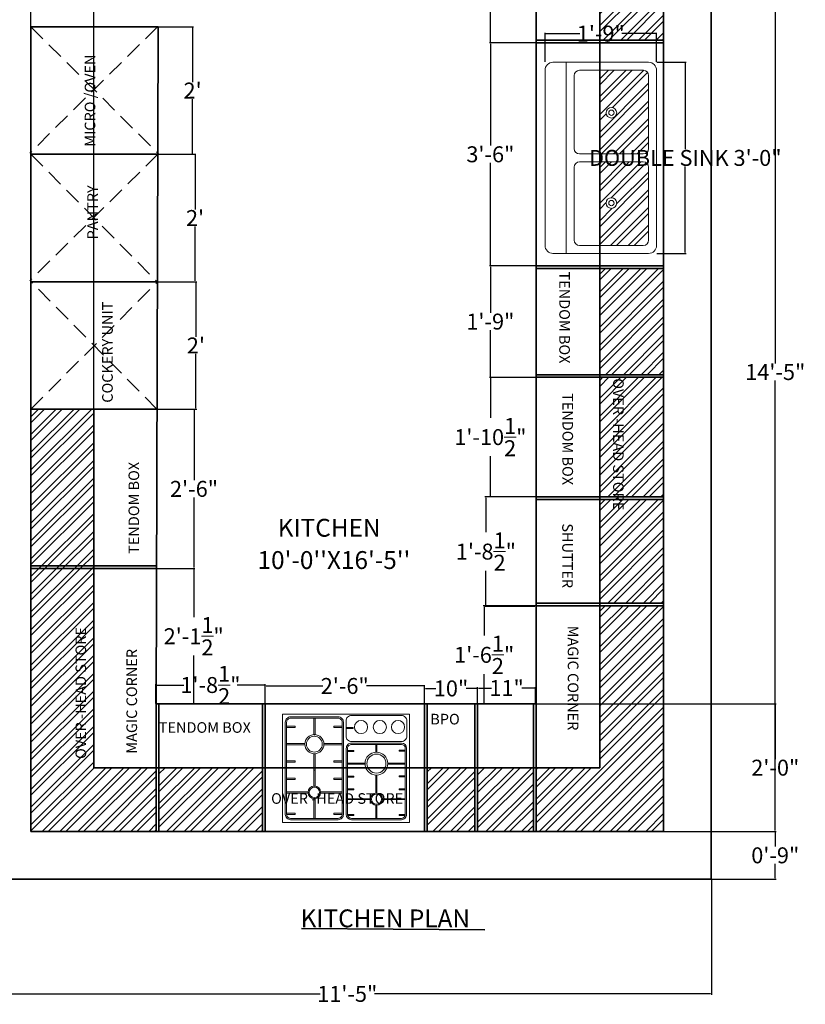
# Model space of a CAD drawing. Units: inches. Extents: x 1686244 to 1686928, y 1936095 to 1936489.
# Tile 7 of 11: x 1686478 to 1686626, y 1936095 to 1936281. Entities that reach past the tile are written whole.
import ezdxf

# ---------------------------------------------------------------- set-up
doc = ezdxf.new("R2010")
doc.units = ezdxf.units.IN
doc.header["$MEASUREMENT"] = 0
doc.linetypes.add('DASHED', pattern=[19.05, 12.7, -6.35])
for name, color, linetype, lineweight in [('A-ANNO-DIMS', 240, 'Continuous', 18), ('A-ANNO-TEXT', 7, 'Continuous', 18), ('A-AREA-IDEN', 3, 'Continuous', 25), ('A-CASE', 7, 'Continuous', 35), ('A-CASE-SWNG', 1, 'DASHED', 18), ('A-FLOR-PATT', 252, 'Continuous', 13), ('A-FURN', 40, 'Continuous', 18)]:
    doc.layers.add(name, color=color, linetype=linetype, lineweight=lineweight)
doc.styles.get("Standard").update_dxf_attribs({"font": 'arial.ttf'})
doc.dimstyles.get("Standard").update_dxf_attribs({"dimtxt": 3, "dimasz": 0.18, "dimexe": 0.18, "dimexo": 0.0625, "dimgap": 0.09, "dimtad": 0, "dimtih": 1, "dimtoh": 1, "dimzin": 0, "dimdsep": 46, "dimlunit": 4, "dimtxsty": 'Standard', "dimcen": 0.09, "dimadec": 0, "dimazin": 0, "dimtfac": 1, "dimtofl": 0, "dimtmove": 0, "dimatfit": 3, "dimfxl": 1, "dimtolj": 1, "dimtzin": 0, "dimarcsym": 0})

# ---------------------------------------------------------------- blocks, each defined once
blk = doc.blocks.new('*D40')
at = {"layer": 'A-ANNO-DIMS', "color": 0, "lineweight": -2, "transparency": 16777216}
for p, q in [((1686503.93, 1936177.36), (1686511.1, 1936177.36)), ((1686510.92, 1936177.18), (1686510.92, 1936168.22)), ((1686510.92, 1936152.04), (1686510.92, 1936161.01)), ((1686503.85, 1936151.86), (1686511.1, 1936151.86))]:
    blk.add_line(p, q, dxfattribs=at)
at = {"layer": 'A-ANNO-DIMS', "color": 0, "transparency": 16777216}
for points in [[(1686510.89, 1936177.18), (1686510.95, 1936177.18), (1686510.92, 1936177.36)], [(1686510.89, 1936152.04), (1686510.95, 1936152.04), (1686510.92, 1936151.86)]]:
    blk.add_solid(points, dxfattribs=at)
at = {"layer": 'Defpoints', "color": 0, "transparency": 16777216}
for p in [(1686503.86, 1936177.36), (1686510.92, 1936177.36), (1686503.79, 1936151.86)]:
    blk.add_point(p, dxfattribs=at)
at = {"layer": 'A-ANNO-DIMS', "color": 0, "transparency": 16777216, "insert": (1686510.92, 1936164.61), "char_height": 3, "attachment_point": 5}
blk.add_mtext('\\A1;2\'-1{\\H1x;\\S1/2;}"', dxfattribs=at)
blk = doc.blocks.new('*D41')
at = {"layer": 'A-ANNO-DIMS', "color": 0, "lineweight": -2, "transparency": 16777216}
for p, q in [((1686503.93, 1936207.36), (1686511.16, 1936207.36)), ((1686510.98, 1936207.18), (1686510.98, 1936193.99)), ((1686510.98, 1936177.54), (1686510.98, 1936190.74)), ((1686503.93, 1936177.36), (1686511.16, 1936177.36))]:
    blk.add_line(p, q, dxfattribs=at)
at = {"layer": 'A-ANNO-DIMS', "color": 0, "transparency": 16777216}
for points in [[(1686510.95, 1936207.18), (1686511.01, 1936207.18), (1686510.98, 1936207.36)], [(1686510.95, 1936177.54), (1686511.01, 1936177.54), (1686510.98, 1936177.36)]]:
    blk.add_solid(points, dxfattribs=at)
at = {"layer": 'Defpoints', "color": 0, "transparency": 16777216}
for p in [(1686503.86, 1936207.36), (1686510.98, 1936207.36), (1686503.86, 1936177.36)]:
    blk.add_point(p, dxfattribs=at)
at = {"layer": 'A-ANNO-DIMS', "color": 0, "transparency": 16777216, "insert": (1686510.98, 1936192.36), "char_height": 3, "attachment_point": 5}
blk.add_mtext('\\A1;2\'-6"', dxfattribs=at)
blk = doc.blocks.new('*D42')
at = {"layer": 'A-ANNO-DIMS', "color": 0, "lineweight": -2, "transparency": 16777216}
for p, q in [((1686504.17, 1936231.36), (1686511.51, 1936231.36)), ((1686511.33, 1936231.18), (1686511.33, 1936220.96)), ((1686511.33, 1936207.54), (1686511.33, 1936217.77)), ((1686503.93, 1936207.36), (1686511.51, 1936207.36))]:
    blk.add_line(p, q, dxfattribs=at)
at = {"layer": 'A-ANNO-DIMS', "color": 0, "transparency": 16777216}
for points in [[(1686511.3, 1936231.18), (1686511.36, 1936231.18), (1686511.33, 1936231.36)], [(1686511.3, 1936207.54), (1686511.36, 1936207.54), (1686511.33, 1936207.36)]]:
    blk.add_solid(points, dxfattribs=at)
at = {"layer": 'Defpoints', "color": 0, "transparency": 16777216}
for p in [(1686504.11, 1936231.36), (1686511.33, 1936231.36), (1686503.86, 1936207.36)]:
    blk.add_point(p, dxfattribs=at)
at = {"layer": 'A-ANNO-DIMS', "color": 0, "transparency": 16777216, "insert": (1686511.33, 1936219.36), "char_height": 3, "attachment_point": 5}
blk.add_mtext("\\A1;2'", dxfattribs=at)
blk = doc.blocks.new('*D43')
at = {"layer": 'A-ANNO-DIMS', "color": 0, "lineweight": -2, "transparency": 16777216}
for p, q in [((1686504.37, 1936255.36), (1686511.35, 1936255.36)), ((1686511.17, 1936255.18), (1686511.17, 1936244.96)), ((1686511.17, 1936231.54), (1686511.17, 1936241.77)), ((1686504.23, 1936231.36), (1686511.35, 1936231.36))]:
    blk.add_line(p, q, dxfattribs=at)
at = {"layer": 'A-ANNO-DIMS', "color": 0, "transparency": 16777216}
for points in [[(1686511.14, 1936255.18), (1686511.2, 1936255.18), (1686511.17, 1936255.36)], [(1686511.14, 1936231.54), (1686511.2, 1936231.54), (1686511.17, 1936231.36)]]:
    blk.add_solid(points, dxfattribs=at)
at = {"layer": 'Defpoints', "color": 0, "transparency": 16777216}
for p in [(1686504.31, 1936255.36), (1686511.17, 1936255.36), (1686504.17, 1936231.36)]:
    blk.add_point(p, dxfattribs=at)
at = {"layer": 'A-ANNO-DIMS', "color": 0, "transparency": 16777216, "insert": (1686511.17, 1936243.36), "char_height": 3, "attachment_point": 5}
blk.add_mtext("\\A1;2'", dxfattribs=at)
blk = doc.blocks.new('*D44')
at = {"layer": 'A-ANNO-DIMS', "color": 0, "lineweight": -2, "transparency": 16777216}
for p, q in [((1686504.19, 1936279.36), (1686510.88, 1936279.36)), ((1686510.7, 1936279.18), (1686510.7, 1936268.96)), ((1686510.7, 1936255.54), (1686510.7, 1936265.77)), ((1686504.19, 1936255.36), (1686510.88, 1936255.36))]:
    blk.add_line(p, q, dxfattribs=at)
at = {"layer": 'A-ANNO-DIMS', "color": 0, "transparency": 16777216}
for points in [[(1686510.67, 1936279.18), (1686510.73, 1936279.18), (1686510.7, 1936279.36)], [(1686510.67, 1936255.54), (1686510.73, 1936255.54), (1686510.7, 1936255.36)]]:
    blk.add_solid(points, dxfattribs=at)
at = {"layer": 'Defpoints', "color": 0, "transparency": 16777216}
for p in [(1686504.12, 1936279.36), (1686510.7, 1936279.36), (1686504.12, 1936255.36)]:
    blk.add_point(p, dxfattribs=at)
at = {"layer": 'A-ANNO-DIMS', "color": 0, "transparency": 16777216, "insert": (1686510.7, 1936267.36), "char_height": 3, "attachment_point": 5}
blk.add_mtext("\\A1;2'", dxfattribs=at)
blk = doc.blocks.new('Sink-double - 36 in top')
for p, q in [((-18, -4), (18, -4)), ((-0.75, -18.5), (-0.75, -6.5)), ((0.75, -6.5), (0.75, -18.5))]:
    blk.add_line(p, q)
for points in [[(-16.5, 0), (16.5, 0)], [(-18, -19.5), (-18, -1.5)], [(18, -1.5), (18, -19.5)], [(-15.5, -5.5), (-1.75, -5.5)], [(1.75, -5.5), (15.5, -5.5)], [(-16.5, -18.5), (-16.5, -6.5)], [(16.5, -6.5), (16.5, -18.5)], [(-1.75, -19.5), (-15.5, -19.5)], [(15.5, -19.5), (1.75, -19.5)], [(16.5, -21), (-16.5, -21)]]:
    blk.add_lwpolyline(points)
for centre, radius in [((-8.5, -12.5), 1), ((-8.5, -12.5), 0.5), ((8.5, -12.5), 1), ((8.5, -12.5), 0.5)]:
    blk.add_circle(centre, radius)
for centre, radius, start, end in [((-16.5, -1.5), 1.5, 90, 180), ((16.5, -1.5), 1.5, 0, 90), ((-15.5, -6.5), 1, 90, 180), ((-1.75, -6.5), 1, 0, 90), ((1.75, -6.5), 1, 90, 180), ((15.5, -6.5), 1, 0, 90), ((-15.5, -18.5), 1, 180, 270), ((-1.75, -18.5), 1, 270, 0), ((1.75, -18.5), 1, 180, 270), ((15.5, -18.5), 1, 270, 0), ((-16.5, -19.5), 1.5, 180, 270), ((16.5, -19.5), 1.5, 270, 0)]:
    blk.add_arc(centre, radius, start, end)
blk = doc.blocks.new('*D46')
at = {"layer": 'A-ANNO-DIMS', "color": 0, "lineweight": -2, "transparency": 16777216}
for p, q in [((1686554.35, 1936151.93), (1686554.35, 1936154.97)), ((1686554.53, 1936154.79), (1686556.51, 1936154.79)), ((1686564.17, 1936154.79), (1686562.18, 1936154.79)), ((1686564.35, 1936151.93), (1686564.35, 1936154.97))]:
    blk.add_line(p, q, dxfattribs=at)
at = {"layer": 'A-ANNO-DIMS', "color": 0, "transparency": 16777216}
for points in [[(1686554.53, 1936154.82), (1686554.53, 1936154.76), (1686554.35, 1936154.79)], [(1686564.17, 1936154.82), (1686564.17, 1936154.76), (1686564.35, 1936154.79)]]:
    blk.add_solid(points, dxfattribs=at)
at = {"layer": 'Defpoints', "color": 0, "transparency": 16777216}
for p in [(1686564.35, 1936154.79), (1686554.35, 1936151.86), (1686564.35, 1936151.86)]:
    blk.add_point(p, dxfattribs=at)
at = {"layer": 'A-ANNO-DIMS', "color": 0, "transparency": 16777216, "insert": (1686559.35, 1936154.79), "char_height": 3, "attachment_point": 5}
blk.add_mtext('\\A1;10"', dxfattribs=at)
blk = doc.blocks.new('*D47')
at = {"layer": 'A-ANNO-DIMS', "color": 0, "lineweight": -2, "transparency": 16777216}
for p, q in [((1686575.28, 1936170.36), (1686565.41, 1936170.36)), ((1686565.59, 1936170.18), (1686565.59, 1936164.74)), ((1686565.59, 1936152.04), (1686565.59, 1936157.49)), ((1686575.28, 1936151.86), (1686565.41, 1936151.86))]:
    blk.add_line(p, q, dxfattribs=at)
at = {"layer": 'A-ANNO-DIMS', "color": 0, "transparency": 16777216}
for points in [[(1686565.56, 1936170.18), (1686565.62, 1936170.18), (1686565.59, 1936170.36)], [(1686565.56, 1936152.04), (1686565.62, 1936152.04), (1686565.59, 1936151.86)]]:
    blk.add_solid(points, dxfattribs=at)
at = {"layer": 'Defpoints', "color": 0, "transparency": 16777216}
for p in [(1686565.59, 1936170.36), (1686575.35, 1936170.36), (1686575.35, 1936151.86)]:
    blk.add_point(p, dxfattribs=at)
at = {"layer": 'A-ANNO-DIMS', "color": 0, "transparency": 16777216, "insert": (1686565.59, 1936161.11), "char_height": 3, "attachment_point": 5}
blk.add_mtext('\\A1;1\'-6{\\H1x;\\S1/2;}"', dxfattribs=at)
blk = doc.blocks.new('*D48')
at = {"layer": 'A-ANNO-DIMS', "color": 0, "lineweight": -2, "transparency": 16777216}
for p, q in [((1686575.28, 1936213.36), (1686566.58, 1936213.36)), ((1686566.76, 1936213.18), (1686566.76, 1936205.74)), ((1686566.76, 1936191.04), (1686566.76, 1936198.49)), ((1686575.16, 1936190.86), (1686566.58, 1936190.86))]:
    blk.add_line(p, q, dxfattribs=at)
at = {"layer": 'A-ANNO-DIMS', "color": 0, "transparency": 16777216}
for points in [[(1686566.73, 1936213.18), (1686566.79, 1936213.18), (1686566.76, 1936213.36)], [(1686566.73, 1936191.04), (1686566.79, 1936191.04), (1686566.76, 1936190.86)]]:
    blk.add_solid(points, dxfattribs=at)
at = {"layer": 'Defpoints', "color": 0, "transparency": 16777216}
for p in [(1686566.76, 1936213.36), (1686575.35, 1936213.36), (1686575.22, 1936190.86)]:
    blk.add_point(p, dxfattribs=at)
at = {"layer": 'A-ANNO-DIMS', "color": 0, "transparency": 16777216, "insert": (1686566.76, 1936202.11), "char_height": 3, "attachment_point": 5}
blk.add_mtext('\\A1;1\'-10{\\H1x;\\S1/2;}"', dxfattribs=at)
blk = doc.blocks.new('*D49')
at = {"layer": 'A-ANNO-DIMS', "color": 0, "lineweight": -2, "transparency": 16777216}
for p, q in [((1686575.28, 1936234.36), (1686566.58, 1936234.36)), ((1686566.76, 1936234.18), (1686566.76, 1936225.49)), ((1686566.76, 1936213.54), (1686566.76, 1936222.24)), ((1686575.28, 1936213.36), (1686566.58, 1936213.36))]:
    blk.add_line(p, q, dxfattribs=at)
at = {"layer": 'A-ANNO-DIMS', "color": 0, "transparency": 16777216}
for points in [[(1686566.73, 1936234.18), (1686566.79, 1936234.18), (1686566.76, 1936234.36)], [(1686566.73, 1936213.54), (1686566.79, 1936213.54), (1686566.76, 1936213.36)]]:
    blk.add_solid(points, dxfattribs=at)
at = {"layer": 'Defpoints', "color": 0, "transparency": 16777216}
for p in [(1686566.76, 1936234.36), (1686575.35, 1936234.36), (1686575.35, 1936213.36)]:
    blk.add_point(p, dxfattribs=at)
at = {"layer": 'A-ANNO-DIMS', "color": 0, "transparency": 16777216, "insert": (1686566.76, 1936223.86), "char_height": 3, "attachment_point": 5}
blk.add_mtext('\\A1;1\'-9"', dxfattribs=at)
blk = doc.blocks.new('*D50')
at = {"layer": 'A-ANNO-DIMS', "color": 0, "lineweight": -2, "transparency": 16777216}
for p, q in [((1686575.28, 1936276.36), (1686566.58, 1936276.36)), ((1686566.76, 1936276.18), (1686566.76, 1936256.99)), ((1686566.76, 1936234.54), (1686566.76, 1936253.74)), ((1686575.28, 1936234.36), (1686566.58, 1936234.36))]:
    blk.add_line(p, q, dxfattribs=at)
at = {"layer": 'A-ANNO-DIMS', "color": 0, "transparency": 16777216}
for points in [[(1686566.73, 1936276.18), (1686566.79, 1936276.18), (1686566.76, 1936276.36)], [(1686566.73, 1936234.54), (1686566.79, 1936234.54), (1686566.76, 1936234.36)]]:
    blk.add_solid(points, dxfattribs=at)
at = {"layer": 'Defpoints', "color": 0, "transparency": 16777216}
for p in [(1686566.76, 1936276.36), (1686575.35, 1936276.36), (1686575.35, 1936234.36)]:
    blk.add_point(p, dxfattribs=at)
at = {"layer": 'A-ANNO-DIMS', "color": 0, "transparency": 16777216, "insert": (1686566.76, 1936255.36), "char_height": 3, "attachment_point": 5}
blk.add_mtext('\\A1;3\'-6"', dxfattribs=at)
blk = doc.blocks.new('*D51')
at = {"layer": 'A-ANNO-DIMS', "color": 0, "lineweight": -2, "transparency": 16777216}
for p, q in [((1686524.35, 1936151.93), (1686524.35, 1936155.43)), ((1686524.53, 1936155.25), (1686535.24, 1936155.25)), ((1686554.17, 1936155.25), (1686543.45, 1936155.25)), ((1686554.35, 1936151.93), (1686554.35, 1936155.43))]:
    blk.add_line(p, q, dxfattribs=at)
at = {"layer": 'A-ANNO-DIMS', "color": 0, "transparency": 16777216}
for points in [[(1686524.53, 1936155.28), (1686524.53, 1936155.22), (1686524.35, 1936155.25)], [(1686554.17, 1936155.28), (1686554.17, 1936155.22), (1686554.35, 1936155.25)]]:
    blk.add_solid(points, dxfattribs=at)
at = {"layer": 'Defpoints', "color": 0, "transparency": 16777216}
for p in [(1686524.35, 1936155.25), (1686524.35, 1936151.86), (1686554.35, 1936151.86)]:
    blk.add_point(p, dxfattribs=at)
at = {"layer": 'A-ANNO-DIMS', "color": 0, "transparency": 16777216, "insert": (1686539.35, 1936155.25), "char_height": 3, "attachment_point": 5}
blk.add_mtext('\\A1;2\'-6"', dxfattribs=at)
blk = doc.blocks.new('*D52')
at = {"layer": 'A-ANNO-DIMS', "color": 0, "lineweight": -2, "transparency": 16777216}
for p, q in [((1686503.79, 1936151.93), (1686503.79, 1936155.61)), ((1686503.97, 1936155.43), (1686509.04, 1936155.43)), ((1686524.17, 1936155.43), (1686519.1, 1936155.43)), ((1686524.35, 1936151.93), (1686524.35, 1936155.61))]:
    blk.add_line(p, q, dxfattribs=at)
at = {"layer": 'A-ANNO-DIMS', "color": 0, "transparency": 16777216}
for points in [[(1686503.97, 1936155.46), (1686503.97, 1936155.4), (1686503.79, 1936155.43)], [(1686524.17, 1936155.46), (1686524.17, 1936155.4), (1686524.35, 1936155.43)]]:
    blk.add_solid(points, dxfattribs=at)
at = {"layer": 'Defpoints', "color": 0, "transparency": 16777216}
for p in [(1686524.35, 1936155.43), (1686503.79, 1936151.86), (1686524.35, 1936151.86)]:
    blk.add_point(p, dxfattribs=at)
at = {"layer": 'A-ANNO-DIMS', "color": 0, "transparency": 16777216, "insert": (1686514.07, 1936155.43), "char_height": 3, "attachment_point": 5}
blk.add_mtext('\\A1;1\'-8{\\H1x;\\S1/2;}"', dxfattribs=at)
blk = doc.blocks.new('*D53')
at = {"layer": 'A-ANNO-DIMS', "color": 0, "lineweight": -2, "transparency": 16777216}
for p, q in [((1686564.35, 1936151.93), (1686564.35, 1936155.04)), ((1686564.53, 1936154.86), (1686566.98, 1936154.86)), ((1686575.1, 1936154.86), (1686572.65, 1936154.86)), ((1686575.28, 1936151.93), (1686575.28, 1936155.04))]:
    blk.add_line(p, q, dxfattribs=at)
at = {"layer": 'A-ANNO-DIMS', "color": 0, "transparency": 16777216}
for points in [[(1686564.53, 1936154.89), (1686564.53, 1936154.83), (1686564.35, 1936154.86)], [(1686575.1, 1936154.89), (1686575.1, 1936154.83), (1686575.28, 1936154.86)]]:
    blk.add_solid(points, dxfattribs=at)
at = {"layer": 'Defpoints', "color": 0, "transparency": 16777216}
for p in [(1686575.28, 1936154.86), (1686564.35, 1936151.86), (1686575.28, 1936151.86)]:
    blk.add_point(p, dxfattribs=at)
at = {"layer": 'A-ANNO-DIMS', "color": 0, "transparency": 16777216, "insert": (1686569.81, 1936154.86), "char_height": 3, "attachment_point": 5}
blk.add_mtext('\\A1;11"', dxfattribs=at)
blk = doc.blocks.new('*D54')
at = {"layer": 'A-ANNO-DIMS', "color": 0, "lineweight": -2, "transparency": 16777216}
for p, q in [((1686575.1, 1936190.86), (1686565.73, 1936190.86)), ((1686565.91, 1936190.68), (1686565.91, 1936184.18)), ((1686565.91, 1936170.42), (1686565.91, 1936176.92)), ((1686575.1, 1936170.24), (1686565.73, 1936170.24))]:
    blk.add_line(p, q, dxfattribs=at)
at = {"layer": 'A-ANNO-DIMS', "color": 0, "transparency": 16777216}
for points in [[(1686565.88, 1936190.68), (1686565.94, 1936190.68), (1686565.91, 1936190.86)], [(1686565.88, 1936170.42), (1686565.94, 1936170.42), (1686565.91, 1936170.24)]]:
    blk.add_solid(points, dxfattribs=at)
at = {"layer": 'Defpoints', "color": 0, "transparency": 16777216}
for p in [(1686575.16, 1936190.86), (1686565.91, 1936170.24), (1686575.16, 1936170.24)]:
    blk.add_point(p, dxfattribs=at)
at = {"layer": 'A-ANNO-DIMS', "color": 0, "transparency": 16777216, "insert": (1686565.91, 1936180.55), "char_height": 3, "attachment_point": 5}
blk.add_mtext('\\A1;1\'-8{\\H1x;\\S1/2;}"', dxfattribs=at)
blk = doc.blocks.new('*D55')
at = {"layer": 'A-ANNO-DIMS', "color": 0, "lineweight": -2, "transparency": 16777216}
for p, q in [((1686575.28, 1936300.86), (1686566.58, 1936300.86)), ((1686566.76, 1936300.68), (1686566.76, 1936292.24)), ((1686566.76, 1936276.54), (1686566.76, 1936284.99)), ((1686575.22, 1936276.36), (1686566.58, 1936276.36))]:
    blk.add_line(p, q, dxfattribs=at)
at = {"layer": 'A-ANNO-DIMS', "color": 0, "transparency": 16777216}
for points in [[(1686566.73, 1936300.68), (1686566.79, 1936300.68), (1686566.76, 1936300.86)], [(1686566.73, 1936276.54), (1686566.79, 1936276.54), (1686566.76, 1936276.36)]]:
    blk.add_solid(points, dxfattribs=at)
at = {"layer": 'Defpoints', "color": 0, "transparency": 16777216}
for p in [(1686566.76, 1936300.86), (1686575.35, 1936300.86), (1686575.28, 1936276.36)]:
    blk.add_point(p, dxfattribs=at)
at = {"layer": 'A-ANNO-DIMS', "color": 0, "transparency": 16777216, "insert": (1686566.76, 1936288.61), "char_height": 3, "attachment_point": 5}
blk.add_mtext('\\A1;2\'-0{\\H1x;\\S1/2;}"', dxfattribs=at)
blk = doc.blocks.new('*D69')
at = {"layer": 'A-ANNO-DIMS', "color": 0, "lineweight": -2, "transparency": 16777216}
for p, q in [((1686598.1, 1936272.68), (1686603.62, 1936272.68)), ((1686603.44, 1936272.5), (1686603.44, 1936256.33)), ((1686603.44, 1936236.86), (1686603.44, 1936253.04)), ((1686598.1, 1936236.68), (1686603.62, 1936236.68))]:
    blk.add_line(p, q, dxfattribs=at)
at = {"layer": 'A-ANNO-DIMS', "color": 0, "transparency": 16777216}
for points in [[(1686603.41, 1936272.5), (1686603.47, 1936272.5), (1686603.44, 1936272.68)], [(1686603.41, 1936236.86), (1686603.47, 1936236.86), (1686603.44, 1936236.68)]]:
    blk.add_solid(points, dxfattribs=at)
at = {"layer": 'Defpoints', "color": 0, "transparency": 16777216}
for p in [(1686598.04, 1936272.68), (1686603.44, 1936272.68), (1686598.04, 1936236.68)]:
    blk.add_point(p, dxfattribs=at)
at = {"layer": 'A-ANNO-DIMS', "color": 0, "transparency": 16777216, "insert": (1686603.44, 1936254.68), "char_height": 3, "attachment_point": 5}
blk.add_mtext('\\A1;DOUBLE SINK 3\'-0"', dxfattribs=at)
blk = doc.blocks.new('*D70')
at = {"layer": 'A-ANNO-DIMS', "color": 0, "lineweight": -2, "transparency": 16777216}
for p, q in [((1686577.04, 1936272.74), (1686577.04, 1936278.26)), ((1686577.22, 1936278.08), (1686583.6, 1936278.08)), ((1686597.86, 1936278.08), (1686591.47, 1936278.08)), ((1686598.04, 1936272.74), (1686598.04, 1936278.26))]:
    blk.add_line(p, q, dxfattribs=at)
at = {"layer": 'A-ANNO-DIMS', "color": 0, "transparency": 16777216}
for points in [[(1686577.22, 1936278.11), (1686577.22, 1936278.05), (1686577.04, 1936278.08)], [(1686597.86, 1936278.11), (1686597.86, 1936278.05), (1686598.04, 1936278.08)]]:
    blk.add_solid(points, dxfattribs=at)
at = {"layer": 'Defpoints', "color": 0, "transparency": 16777216}
for p in [(1686577.04, 1936278.08), (1686577.04, 1936272.68), (1686598.04, 1936272.68)]:
    blk.add_point(p, dxfattribs=at)
at = {"layer": 'A-ANNO-DIMS', "color": 0, "transparency": 16777216, "insert": (1686587.54, 1936278.08), "char_height": 3, "attachment_point": 5}
blk.add_mtext('\\A1;1\'-9"', dxfattribs=at)
blk = doc.blocks.new('*D113')
at = {"layer": 'A-ANNO-DIMS', "color": 0, "lineweight": -2, "transparency": 16777216}
for p, q in [((1686471.29, 1936118.8), (1686471.29, 1936097.09)), ((1686608.35, 1936118.8), (1686608.35, 1936097.09)), ((1686471.47, 1936097.27), (1686534.72, 1936097.27)), ((1686608.17, 1936097.27), (1686544.92, 1936097.27))]:
    blk.add_line(p, q, dxfattribs=at)
at = {"layer": 'A-ANNO-DIMS', "color": 0, "transparency": 16777216}
for points in [[(1686471.47, 1936097.3), (1686471.47, 1936097.24), (1686471.29, 1936097.27)], [(1686608.17, 1936097.3), (1686608.17, 1936097.24), (1686608.35, 1936097.27)]]:
    blk.add_solid(points, dxfattribs=at)
at = {"layer": 'Defpoints', "color": 0, "transparency": 16777216}
for p in [(1686471.29, 1936118.86), (1686608.35, 1936118.86), (1686608.35, 1936097.27)]:
    blk.add_point(p, dxfattribs=at)
at = {"layer": 'A-ANNO-DIMS', "color": 0, "transparency": 16777216, "insert": (1686539.82, 1936097.27), "char_height": 3, "attachment_point": 5}
blk.add_mtext('\\A1;11\'-5"', dxfattribs=at)
blk = doc.blocks.new('*D115')
at = {"layer": 'A-ANNO-DIMS', "color": 0, "lineweight": -2, "transparency": 16777216}
for p, q in [((1686599.41, 1936127.86), (1686620.56, 1936127.86)), ((1686620.38, 1936127.68), (1686620.38, 1936124.99)), ((1686620.38, 1936119.04), (1686620.38, 1936121.74)), ((1686608.41, 1936118.86), (1686620.56, 1936118.86))]:
    blk.add_line(p, q, dxfattribs=at)
at = {"layer": 'A-ANNO-DIMS', "color": 0, "transparency": 16777216}
for points in [[(1686620.35, 1936127.68), (1686620.41, 1936127.68), (1686620.38, 1936127.86)], [(1686620.35, 1936119.04), (1686620.41, 1936119.04), (1686620.38, 1936118.86)]]:
    blk.add_solid(points, dxfattribs=at)
at = {"layer": 'Defpoints', "color": 0, "transparency": 16777216}
for p in [(1686599.35, 1936127.86), (1686620.38, 1936127.86), (1686608.35, 1936118.86)]:
    blk.add_point(p, dxfattribs=at)
at = {"layer": 'A-ANNO-DIMS', "color": 0, "transparency": 16777216, "insert": (1686620.38, 1936123.36), "char_height": 3, "attachment_point": 5}
blk.add_mtext('\\A1;0\'-9"', dxfattribs=at)
blk = doc.blocks.new('*D116')
at = {"layer": 'A-ANNO-DIMS', "color": 0, "lineweight": -2, "transparency": 16777216}
for p, q in [((1686480.29, 1936207.43), (1686480.29, 1936353.25)), ((1686480.47, 1936353.07), (1686482.26, 1936353.07)), ((1686491.93, 1936353.07), (1686490.14, 1936353.07)), ((1686492.11, 1936207.43), (1686492.11, 1936353.25))]:
    blk.add_line(p, q, dxfattribs=at)
at = {"layer": 'A-ANNO-DIMS', "color": 0, "transparency": 16777216}
for points in [[(1686480.47, 1936353.1), (1686480.47, 1936353.04), (1686480.29, 1936353.07)], [(1686491.93, 1936353.1), (1686491.93, 1936353.04), (1686492.11, 1936353.07)]]:
    blk.add_solid(points, dxfattribs=at)
at = {"layer": 'Defpoints', "color": 0, "transparency": 16777216}
for p in [(1686492.11, 1936353.07), (1686480.29, 1936207.36), (1686492.11, 1936207.36)]:
    blk.add_point(p, dxfattribs=at)
at = {"layer": 'A-ANNO-DIMS', "color": 0, "transparency": 16777216, "insert": (1686486.2, 1936353.07), "char_height": 3, "attachment_point": 5}
blk.add_mtext('\\A1;1\'-0"', dxfattribs=at)
blk = doc.blocks.new('*D119')
at = {"layer": 'A-ANNO-DIMS', "color": 0, "lineweight": -2, "transparency": 16777216}
for p, q in [((1686575.41, 1936151.86), (1686620.56, 1936151.86)), ((1686620.38, 1936151.68), (1686620.38, 1936141.49)), ((1686620.38, 1936128.04), (1686620.38, 1936138.24)), ((1686575.41, 1936127.86), (1686620.56, 1936127.86))]:
    blk.add_line(p, q, dxfattribs=at)
at = {"layer": 'A-ANNO-DIMS', "color": 0, "transparency": 16777216}
for points in [[(1686620.35, 1936151.68), (1686620.41, 1936151.68), (1686620.38, 1936151.86)], [(1686620.35, 1936128.04), (1686620.41, 1936128.04), (1686620.38, 1936127.86)]]:
    blk.add_solid(points, dxfattribs=at)
at = {"layer": 'Defpoints', "color": 0, "transparency": 16777216}
for p in [(1686575.35, 1936151.86), (1686620.38, 1936151.86), (1686575.35, 1936127.86)]:
    blk.add_point(p, dxfattribs=at)
at = {"layer": 'A-ANNO-DIMS', "color": 0, "transparency": 16777216, "insert": (1686620.38, 1936139.86), "char_height": 3, "attachment_point": 5}
blk.add_mtext('\\A1;2\'-0"', dxfattribs=at)
blk = doc.blocks.new('*D120')
at = {"layer": 'A-ANNO-DIMS', "color": 0, "lineweight": -2, "transparency": 16777216}
for p, q in [((1686599.41, 1936300.86), (1686620.56, 1936300.86)), ((1686620.38, 1936300.68), (1686620.38, 1936215.99)), ((1686620.38, 1936128.04), (1686620.38, 1936212.74)), ((1686599.41, 1936127.86), (1686620.56, 1936127.86))]:
    blk.add_line(p, q, dxfattribs=at)
at = {"layer": 'A-ANNO-DIMS', "color": 0, "transparency": 16777216}
for points in [[(1686620.35, 1936300.68), (1686620.41, 1936300.68), (1686620.38, 1936300.86)], [(1686620.35, 1936128.04), (1686620.41, 1936128.04), (1686620.38, 1936127.86)]]:
    blk.add_solid(points, dxfattribs=at)
at = {"layer": 'Defpoints', "color": 0, "transparency": 16777216}
for p in [(1686599.35, 1936300.86), (1686599.35, 1936127.86), (1686620.38, 1936127.86)]:
    blk.add_point(p, dxfattribs=at)
at = {"layer": 'A-ANNO-DIMS', "color": 0, "transparency": 16777216, "insert": (1686620.38, 1936214.36), "char_height": 3, "attachment_point": 5}
blk.add_mtext('\\A1;14\'-5"', dxfattribs=at)

msp = doc.modelspace()

# ---------------------------------------------------------------- hatches: boundary and pattern name
at = {"layer": 'A-FLOR-PATT'}
h = msp.add_hatch(dxfattribs=at)
h.set_pattern_fill('ANSI32', color=256, scale=6.3)
h.paths.add_polyline_path([(1686599.345, 1936233.864), (1686587.345, 1936233.864), (1686587.345, 1936213.864), (1686599.345, 1936213.864)])
h.paths.add_polyline_path([(1686596.539, 1936252.932, 0.4142136), (1686595.539, 1936253.932), (1686587.345, 1936253.932), (1686587.345, 1936238.182), (1686595.539, 1936238.182, 0.4142136), (1686596.539, 1936239.182)])
h.paths.add_polyline_path([(1686590.539, 1936246.182, -1), (1686588.539, 1936246.182, -1)], flags=16)
h.paths.add_polyline_path([(1686590.039, 1936246.182, -1), (1686589.039, 1936246.182, -1)], flags=0)
h.paths.add_polyline_path([(1686599.345, 1936300.364), (1686587.345, 1936300.364), (1686587.345, 1936276.864), (1686599.345, 1936276.864)])
h.paths.add_polyline_path([(1686596.539, 1936270.182, 0.4142136), (1686595.539, 1936271.182), (1686587.345, 1936271.182), (1686587.345, 1936255.432), (1686595.539, 1936255.432, 0.4142136), (1686596.539, 1936256.432)])
h.paths.add_polyline_path([(1686590.539, 1936263.182, -1), (1686588.539, 1936263.182, -1)], flags=16)
h.paths.add_polyline_path([(1686589.039, 1936263.182, -1), (1686590.039, 1936263.182, -1)], flags=0)
h = msp.add_hatch(dxfattribs=at)
h.set_pattern_fill('ANSI32', color=256, scale=6.3)
h.paths.add_polyline_path([(1686504.349, 1936139.864), (1686504.349, 1936127.864), (1686523.845, 1936127.864), (1686523.845, 1936139.864)])
h.paths.add_polyline_path([(1686563.845, 1936139.864), (1686554.845, 1936139.864), (1686554.845, 1936127.864), (1686563.845, 1936127.864)])
h.paths.add_polyline_path([(1686574.845, 1936139.864), (1686564.345, 1936139.864), (1686564.345, 1936127.864), (1686574.845, 1936127.864)])
h.paths.add_polyline_path([(1686599.345, 1936127.864), (1686599.345, 1936151.864), (1686599.345, 1936170.364), (1686587.345, 1936170.364), (1686587.345, 1936139.864), (1686575.345, 1936139.864), (1686575.345, 1936127.864)])
h.paths.add_polyline_path([(1686587.345, 1936170.864), (1686599.345, 1936170.864), (1686599.345, 1936190.364), (1686587.345, 1936190.364)])
h.paths.add_polyline_path([(1686599.345, 1936190.864), (1686599.345, 1936213.364), (1686587.345, 1936213.364), (1686587.345, 1936190.864)])
h.paths.add_polyline_path([(1686524.971, 1936132.506), (1686553.794, 1936132.506), (1686553.794, 1936135.611), (1686524.971, 1936135.611)], flags=9)
h.paths.add_polyline_path([(1686589.299, 1936213.706), (1686589.299, 1936184.883), (1686592.403, 1936184.883), (1686592.403, 1936213.706)], flags=9)
h = msp.add_hatch(dxfattribs=at)
h.set_pattern_fill('ANSI32', color=256, scale=6.3)
h.paths.add_polyline_path([(1686480.291, 1936177.363), (1686492.108, 1936177.363), (1686492.108, 1936207.363), (1686480.291, 1936207.363)])
h = msp.add_hatch(dxfattribs=at)
h.set_pattern_fill('ANSI32', color=256, scale=6.3)
h.paths.add_polyline_path([(1686503.849, 1936127.864), (1686503.849, 1936139.864), (1686492.108, 1936139.864), (1686492.108, 1936177.363), (1686480.291, 1936177.363), (1686480.291, 1936127.864)])
h.paths.add_polyline_path([(1686491.226, 1936140.985), (1686491.226, 1936169.809), (1686488.122, 1936169.809), (1686488.122, 1936140.985)], flags=24)

# ---------------------------------------------------------------- linework, layer by layer
at = {"layer": 'A-CASE'}
for p, q in [((1686587.345, 1936139.864), (1686587.345, 1936300.364)), ((1686504.227, 1936279.362), (1686480.291, 1936279.362)), ((1686504.227, 1936279.362), (1686504.2, 1936279.362)), ((1686575.345, 1936276.864), (1686599.345, 1936276.864)), ((1686575.345, 1936276.364), (1686599.345, 1936276.364)), ((1686504.157, 1936255.364), (1686480.291, 1936255.362)), ((1686575.345, 1936234.364), (1686599.345, 1936234.364)), ((1686575.345, 1936233.864), (1686599.345, 1936233.864)), ((1686504.086, 1936231.362), (1686480.291, 1936231.362)), ((1686575.345, 1936213.864), (1686599.345, 1936213.864)), ((1686575.345, 1936213.364), (1686599.345, 1936213.364)), ((1686503.924, 1936207.363), (1686480.291, 1936207.363)), ((1686492.108, 1936207.363), (1686492.108, 1936139.864)), ((1686575.345, 1936190.864), (1686599.345, 1936190.864)), ((1686575.345, 1936190.364), (1686599.345, 1936190.364)), ((1686503.862, 1936177.863), (1686480.291, 1936177.863)), ((1686503.862, 1936177.363), (1686480.291, 1936177.363)), ((1686575.345, 1936170.864), (1686599.345, 1936170.864)), ((1686575.345, 1936170.364), (1686599.345, 1936170.364)), ((1686503.85, 1936151.863), (1686503.849, 1936127.864)), ((1686575.345, 1936151.864), (1686503.85, 1936151.863)), ((1686504.35, 1936151.863), (1686504.349, 1936127.864)), ((1686523.845, 1936151.864), (1686523.845, 1936127.864)), ((1686524.345, 1936151.864), (1686524.345, 1936127.864)), ((1686554.345, 1936151.864), (1686554.345, 1936127.864)), ((1686554.845, 1936151.864), (1686554.845, 1936127.864)), ((1686563.845, 1936151.864), (1686563.845, 1936127.864)), ((1686564.345, 1936151.864), (1686564.345, 1936127.864)), ((1686574.845, 1936151.864), (1686574.845, 1936127.864)), ((1686575.345, 1936151.864), (1686575.345, 1936127.864)), ((1686587.345, 1936139.864), (1686492.108, 1936139.864)), ((1686565.725, 1936109.305), (1686531.176, 1936109.575))]:
    msp.add_line(p, q, dxfattribs=at)
for points in [[(1686608.345, 1936303.497), (1686608.345, 1936118.864), (1686471.291, 1936118.864), (1686471.291, 1936321.159)], [(1686503.85, 1936151.863), (1686524.345, 1936151.864), (1686554.345, 1936151.864), (1686564.345, 1936151.864), (1686575.345, 1936151.864), (1686575.345, 1936170.364), (1686575.345, 1936190.864), (1686575.345, 1936213.364), (1686575.345, 1936234.364), (1686575.345, 1936276.364), (1686575.345, 1936300.864), (1686599.345, 1936300.864), (1686599.345, 1936151.864), (1686599.345, 1936127.864), (1686504.291, 1936127.864), (1686480.291, 1936127.864), (1686480.291, 1936279.362)], [(1686504.2, 1936279.362), (1686503.85, 1936151.863)]]:
    msp.add_lwpolyline(points, dxfattribs=at)
at = {"layer": 'A-CASE-SWNG', "ltscale": 0.25}
for p, q in [((1686504.123, 1936279.362), (1686480.077, 1936255.578)), ((1686480.291, 1936279.362), (1686504.374, 1936255.362)), ((1686504.186, 1936255.362), (1686480.095, 1936231.561)), ((1686480.291, 1936255.362), (1686504.068, 1936231.322)), ((1686480.291, 1936207.363), (1686504.107, 1936231.362)), ((1686504.002, 1936207.363), (1686480.291, 1936231.362))]:
    msp.add_line(p, q, dxfattribs=at)
at = {"layer": 'A-FURN'}
for points in [[(1686527.661, 1936149.925), (1686551.534, 1936149.925), (1686551.534, 1936129.57), (1686527.661, 1936129.57)], [(1686533.509, 1936149.175), (1686533.75, 1936149.175), (1686533.75, 1936146.078), (1686533.509, 1936146.078)], [(1686528.411, 1936147.682), (1686529.994, 1936147.682), (1686529.994, 1936147.432), (1686528.411, 1936147.432)], [(1686538.848, 1936147.682), (1686537.265, 1936147.682), (1686537.265, 1936147.432), (1686538.848, 1936147.432)], [(1686539.741, 1936147.436), (1686540.91, 1936147.436), (1686540.91, 1936147.252), (1686539.741, 1936147.252)], [(1686528.411, 1936144.409), (1686531.836, 1936144.409), (1686531.836, 1936144.16), (1686528.411, 1936144.16)], [(1686538.848, 1936144.409), (1686535.423, 1936144.409), (1686535.423, 1936144.16), (1686538.848, 1936144.16)], [(1686545.225, 1936144.244), (1686545.403, 1936144.244), (1686545.403, 1936142.784), (1686545.225, 1936142.784)], [(1686533.509, 1936139.394), (1686533.75, 1936139.394), (1686533.75, 1936142.491), (1686533.509, 1936142.491)], [(1686539.892, 1936143.1), (1686541.061, 1936143.1), (1686541.061, 1936142.916), (1686539.892, 1936142.916)], [(1686550.743, 1936143.142), (1686549.574, 1936143.142), (1686549.574, 1936142.958), (1686550.743, 1936142.958)], [(1686528.411, 1936141.137), (1686529.994, 1936141.137), (1686529.994, 1936140.888), (1686528.411, 1936140.888)], [(1686538.848, 1936141.137), (1686537.265, 1936141.137), (1686537.265, 1936140.888), (1686538.848, 1936140.888)], [(1686539.878, 1936140.724), (1686543.162, 1936140.724), (1686543.162, 1936140.54), (1686539.878, 1936140.54)], [(1686550.75, 1936140.724), (1686547.465, 1936140.724), (1686547.465, 1936140.54), (1686550.75, 1936140.54)], [(1686533.509, 1936139.394), (1686533.75, 1936139.394), (1686533.75, 1936136.38), (1686533.509, 1936136.38)], [(1686528.411, 1936137.864), (1686529.994, 1936137.864), (1686529.994, 1936137.615), (1686528.411, 1936137.615)], [(1686538.848, 1936137.864), (1686537.265, 1936137.864), (1686537.265, 1936137.615), (1686538.848, 1936137.615)], [(1686539.892, 1936138.267), (1686541.061, 1936138.267), (1686541.061, 1936138.083), (1686539.892, 1936138.083)], [(1686545.225, 1936137.021), (1686545.403, 1936137.021), (1686545.403, 1936138.481), (1686545.225, 1936138.481)], [(1686545.225, 1936137.021), (1686545.403, 1936137.021), (1686545.403, 1936135.085), (1686545.225, 1936135.085)], [(1686550.743, 1936138.309), (1686549.574, 1936138.309), (1686549.574, 1936138.125), (1686550.743, 1936138.125)], [(1686528.411, 1936135.086), (1686532.46, 1936135.086), (1686532.46, 1936135.335), (1686528.411, 1936135.335)], [(1686538.848, 1936135.086), (1686534.799, 1936135.086), (1686534.799, 1936135.335), (1686538.848, 1936135.335)], [(1686539.892, 1936135.851), (1686541.061, 1936135.851), (1686541.061, 1936135.667), (1686539.892, 1936135.667)], [(1686550.743, 1936135.892), (1686549.574, 1936135.892), (1686549.574, 1936135.708), (1686550.743, 1936135.708)], [(1686533.509, 1936130.32), (1686533.75, 1936130.32), (1686533.75, 1936134.042), (1686533.509, 1936134.042)], [(1686539.878, 1936133.84), (1686544.161, 1936133.84), (1686544.161, 1936134.024), (1686539.878, 1936134.024)], [(1686550.75, 1936133.84), (1686546.467, 1936133.84), (1686546.467, 1936134.024), (1686550.75, 1936134.024)], [(1686528.411, 1936131.319), (1686529.994, 1936131.319), (1686529.994, 1936131.07), (1686528.411, 1936131.07)], [(1686538.848, 1936131.319), (1686537.265, 1936131.319), (1686537.265, 1936131.07), (1686538.848, 1936131.07)], [(1686545.225, 1936130.32), (1686545.403, 1936130.32), (1686545.403, 1936132.779), (1686545.225, 1936132.779)], [(1686539.892, 1936131.018), (1686541.061, 1936131.018), (1686541.061, 1936130.833), (1686539.892, 1936130.833)], [(1686550.743, 1936131.059), (1686549.574, 1936131.059), (1686549.574, 1936130.875), (1686550.743, 1936130.875)]]:
    msp.add_lwpolyline(points, close=True, dxfattribs=at)
for points in [[(1686540.598, 1936149.696), (1686550.034, 1936149.696, -0.4142136), (1686551.034, 1936148.696), (1686551.034, 1936145.797, -0.4142136), (1686550.034, 1936144.797), (1686540.598, 1936144.797, -0.4142136), (1686539.598, 1936145.797), (1686539.598, 1936148.696, -0.4142136)], [(1686538.098, 1936130.07), (1686529.161, 1936130.07, -0.4142136), (1686528.161, 1936131.07), (1686528.161, 1936148.425, -0.4142136), (1686529.161, 1936149.425), (1686538.098, 1936149.425, -0.4142136), (1686539.098, 1936148.425), (1686539.098, 1936131.07, -0.4142136)], [(1686538.098, 1936130.32), (1686529.161, 1936130.32, -0.4142136), (1686528.411, 1936131.07), (1686528.411, 1936148.425, -0.4142136), (1686529.161, 1936149.175), (1686538.098, 1936149.175, -0.4142136), (1686538.848, 1936148.425), (1686538.848, 1936131.07, -0.4142136)], [(1686540.628, 1936144.494), (1686550, 1936144.494, -0.4142094), (1686551, 1936143.494), (1686551, 1936131.07, -0.4142177), (1686550, 1936130.07), (1686540.628, 1936130.07, -0.4142094), (1686539.628, 1936131.07), (1686539.628, 1936143.494, -0.4142177)], [(1686540.628, 1936144.244), (1686550, 1936144.244, -0.4142094), (1686550.75, 1936143.494), (1686550.75, 1936131.07, -0.4142177), (1686550, 1936130.32), (1686540.628, 1936130.32, -0.4142094), (1686539.878, 1936131.07), (1686539.878, 1936143.494, -0.4142177)]]:
    msp.add_lwpolyline(points, format="xyb", close=True, dxfattribs=at)
for centre, radius in [((1686542.417, 1936147.514), 1.242), ((1686545.952, 1936147.514), 1.242), ((1686549.376, 1936147.514), 1.242), ((1686533.63, 1936144.285), 1.794), ((1686533.63, 1936144.285), 1.496), ((1686545.314, 1936140.632), 2.152), ((1686545.314, 1936140.632), 1.795), ((1686533.63, 1936135.211), 1.169), ((1686533.63, 1936135.211), 0.975), ((1686545.314, 1936133.932), 1.153), ((1686545.314, 1936133.932), 0.962)]:
    msp.add_circle(centre, radius, dxfattribs=at)

# ---------------------------------------------------------------- block references
at = {"layer": 'A-FURN', "rotation": 90}
msp.add_blockref('Sink-double - 36 in top', (1686577.039, 1936254.682), dxfattribs=at)

# ---------------------------------------------------------------- texts
at = {"layer": 'A-ANNO-TEXT'}
for s, rotation, p in [('MICRO /OVEN', 90, (1686492.404, 1936256.787)), ('PANTRY', 90, (1686492.889, 1936239.34)), ('TENDOM BOX', 269.96854, (1686579.732, 1936233.293)), ('COCKERY UNIT', 90, (1686495.684, 1936208.58)), ('OVER -HEAD STORE', 270, (1686589.851, 1936213.189)), ('TENDOM BOX', 269.96854, (1686580.323, 1936210.396)), ('TENDOM BOX', 90, (1686500.649, 1936180.126)), ('SHUTTER', 269.96854, (1686580.282, 1936185.862)), ('MAGIC CORNER', 270, (1686581.326, 1936166.592)), ('OVER -HEAD STORE', 90, (1686490.675, 1936141.503)), ('MAGIC CORNER', 90, (1686500.256, 1936142.5))]:
    msp.add_text(s, height=2, rotation=rotation, dxfattribs=at).set_placement(p)
for s, height, p in [('BPO', 2, (1686555.45, 1936148.002)), ('TENDOM BOX', 2, (1686504.35, 1936146.43)), ('OVER -HEAD STORE', 2, (1686525.488, 1936133.058)), ('KITCHEN PLAN', 3.36498, (1686531.037, 1936109.806))]:
    msp.add_text(s, height=height, dxfattribs=at).set_placement(p)
at = {"layer": 'A-AREA-IDEN'}
for s, height, p in [('KITCHEN', 3.365, (1686526.732, 1936183.354)), ("10'-0''X16'-5''", 3.36498, (1686522.934, 1936177.276))]:
    msp.add_text(s, height=height, dxfattribs=at).set_placement(p)

# ---------------------------------------------------------------- dimensions: what is measured, and where the dimension line sits
at = {"layer": 'A-ANNO-DIMS'}
for base, p1, p2, override, picture, middle in [((1686492.108, 1936353.067), (1686480.291, 1936207.363), (1686492.108, 1936207.363), {"dimdec": 1, "dimlfac": 1, "dimrnd": 0, "dimzin": 1, "dimdsep": 46, "dimlunit": 4, "dimfrac": 2}, '*D116', (1686486.2, 1936353.067)), ((1686524.345, 1936155.428), (1686503.788, 1936151.863), (1686524.345, 1936151.863), {"dimclrd": 0, "dimclre": 0, "dimclrt": 0}, '*D52', (1686514.066, 1936155.428)), ((1686524.345, 1936155.248), (1686554.345, 1936151.864), (1686524.345, 1936151.864), {"dimclrd": 0, "dimclre": 0, "dimclrt": 0}, '*D51', (1686539.345, 1936155.248)), ((1686564.345, 1936154.786), (1686554.345, 1936151.864), (1686564.345, 1936151.864), {"dimclrd": 0, "dimclre": 0, "dimclrt": 0}, '*D46', (1686559.345, 1936154.786)), ((1686575.283, 1936154.857), (1686564.345, 1936151.864), (1686575.283, 1936151.864), {"dimclrd": 0, "dimclre": 0, "dimclrt": 0}, '*D53', (1686569.814, 1936154.857)), ((1686608.345, 1936097.275), (1686471.291, 1936118.864), (1686608.345, 1936118.864), {"dimdec": 1, "dimlfac": 1, "dimrnd": 0, "dimzin": 1, "dimdsep": 46, "dimlunit": 4, "dimfrac": 2}, '*D113', (1686539.818, 1936097.275))]:
    dim = msp.add_linear_dim(base=base, p1=p1, p2=p2, dimstyle='Standard', override=override, dxfattribs=at)
    dim.commit()
    dim.dimension.update_dxf_attribs({"geometry": picture, "text_midpoint": middle})
for base, p1, p2, angle, override, picture, middle in [((1686566.76, 1936300.864), (1686575.283, 1936276.364), (1686575.345, 1936300.864), 90, {"dimclrd": 0, "dimclre": 0, "dimclrt": 0}, '*D55', (1686566.76, 1936288.614)), ((1686620.375, 1936127.864), (1686599.345, 1936300.864), (1686599.345, 1936127.864), 90, {"dimdec": 1, "dimlfac": 1, "dimrnd": 0, "dimzin": 1, "dimdsep": 46, "dimlunit": 4, "dimfrac": 2}, '*D120', (1686620.375, 1936214.364)), ((1686577.039, 1936278.082), (1686598.039, 1936272.682), (1686577.039, 1936272.682), 180, {"dimdec": 1, "dimrnd": 0, "dimzin": 1, "dimlunit": 4, "dimfrac": 2}, '*D70', (1686587.539, 1936278.082)), ((1686566.76, 1936276.364), (1686575.345, 1936234.364), (1686575.345, 1936276.364), 90, {"dimclrd": 0, "dimclre": 0, "dimclrt": 0}, '*D50', (1686566.76, 1936255.364)), ((1686566.76, 1936234.364), (1686575.345, 1936213.364), (1686575.345, 1936234.364), 90, {"dimclrd": 0, "dimclre": 0, "dimclrt": 0}, '*D49', (1686566.76, 1936223.864)), ((1686566.76, 1936213.364), (1686575.22, 1936190.864), (1686575.345, 1936213.364), 90, {"dimclrd": 0, "dimclre": 0, "dimclrt": 0}, '*D48', (1686566.76, 1936202.114)), ((1686565.912877926, 1936170.239199435), (1686575.157780409, 1936190.864199433), (1686575.157780409, 1936170.239199434), 90, {"dimclrd": 0, "dimclre": 0, "dimclrt": 0}, '*D54', (1686565.912877926, 1936180.551699433)), ((1686620.375, 1936151.864), (1686575.345, 1936127.864), (1686575.345, 1936151.864), 90, {"dimdec": 1, "dimlfac": 1, "dimrnd": 0, "dimzin": 1, "dimdsep": 46, "dimlunit": 4, "dimfrac": 2}, '*D119', (1686620.375, 1936139.864)), ((1686620.375, 1936127.864), (1686608.345, 1936118.864), (1686599.345, 1936127.864), 90, {"dimdec": 1, "dimlfac": 1, "dimrnd": 0, "dimzin": 1, "dimdsep": 46, "dimlunit": 4, "dimfrac": 2}, '*D115', (1686620.375, 1936123.364))]:
    dim = msp.add_linear_dim(base=base, p1=p1, p2=p2, angle=angle, dimstyle='Standard', override=override, dxfattribs=at)
    dim.commit()
    dim.dimension.update_dxf_attribs({"geometry": picture, "text_midpoint": middle})
for base, p1, p2, picture, middle in [((1686510.696, 1936279.362), (1686504.123, 1936255.362), (1686504.123, 1936279.362), '*D44', (1686510.696, 1936267.362)), ((1686511.169, 1936255.362), (1686504.17, 1936231.362), (1686504.312, 1936255.362), '*D43', (1686511.169, 1936243.362)), ((1686511.329, 1936231.362), (1686503.863, 1936207.363), (1686504.107, 1936231.362), '*D42', (1686511.329, 1936219.363)), ((1686510.984, 1936207.363), (1686503.863, 1936177.363), (1686503.863, 1936207.363), '*D41', (1686510.984, 1936192.363)), ((1686510.922, 1936177.363), (1686503.788, 1936151.863), (1686503.863, 1936177.363), '*D40', (1686510.922, 1936164.613)), ((1686565.594, 1936170.364), (1686575.345, 1936151.864), (1686575.345, 1936170.364), '*D47', (1686565.594, 1936161.114))]:
    dim = msp.add_linear_dim(base=base, p1=p1, p2=p2, angle=90, dimstyle='Standard', override={"dimclrd": 0, "dimclre": 0, "dimclrt": 0}, dxfattribs=at)
    dim.commit()
    dim.dimension.update_dxf_attribs({"geometry": picture, "text_midpoint": middle, "dimtype": 160})
dim = msp.add_linear_dim(base=(1686603.439, 1936272.682), p1=(1686598.039, 1936236.682), p2=(1686598.039, 1936272.682), angle=90, text='DOUBLE SINK <>', dimstyle='Standard', override={"dimdec": 1, "dimrnd": 0, "dimzin": 1, "dimlunit": 4, "dimfrac": 2}, dxfattribs=at)
dim.commit()
dim.dimension.update_dxf_attribs({"geometry": '*D69', "text_midpoint": (1686603.439, 1936254.682)})

doc.saveas('drawing.dxf')
